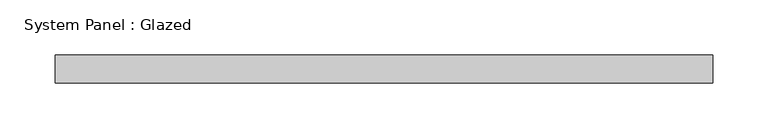
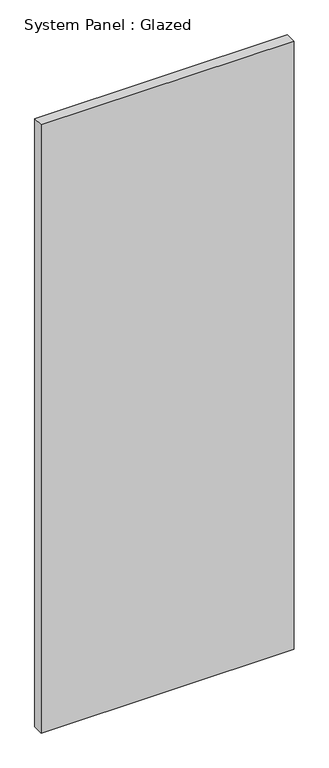
"""IFC4 building model written with IfcOpenShell, lengths in millimetres: plate geometry, System Panel : Glazed."""

from ifc_helpers import new_model, si_unit, origin, origin_with_axes, place, context, project, spatial, polyline, outline, extrude, source, transform, mapped, element, save


def system_panel_glazed_3427ea54(model_context):
    return source(origin(), model_context, "Body", "SweptSolid", [
        extrude(outline(polyline([(298.45, 19.05), (-298.45, 19.05), (-298.45, 44.45), (298.45, 44.45), (298.45, 19.05)])), origin_with_axes(), (0.0, 0.0, 1.0), 1516.8504197),
    ])


if __name__ == "__main__":
    model = new_model("IFC4")
    model_context = context("Model", 3, world=origin())
    ifc_project = project(units=[si_unit("LENGTHUNIT", "METRE", prefix="MILLI")], contexts=[model_context])
    site = spatial("IfcSite", under=ifc_project)
    building = spatial("IfcBuilding", under=site)
    placement = place(None, origin())
    system_panel_glazed_shape = system_panel_glazed_3427ea54(model_context)
    element("IfcPlate", 1, ObjectType="System Panel : Glazed", at=placement, inside=building, context=model_context, shape_type="MappedRepresentation", body=[
        mapped(system_panel_glazed_shape, transform((0.0, 0.0, 0.0), x_axis=(1.0, 0.0, 0.0), y_axis=(0.0, 1.0, 0.0), z_axis=(0.0, 0.0, 1.0))),
    ])
    save(model, "model.ifc")

# Revit data of these elements
# Type "System Panel : Glazed"
#   Construction Type Id = "GSP4R"
#   Analytic Construction = "1/8 in Pilkington single glazing"
#   Visual Light Transmittance = 0.9
#   Solar Heat Gain Coefficient = 0.86
#   Heat Transfer Coefficient (U) = 1.18115 BTU/(h·ft²·°F)
#   Define Thermal Properties by = 1
# Element 1 (IfcPlate, "System Panel : Glazed")
#   Materials on its faces: "Glass"
# Materials
#   "Glass": class "Glass", colour RGB 0 128 192, transparency 0.75, Description = "Soda Lime Glass", Cost = 0
